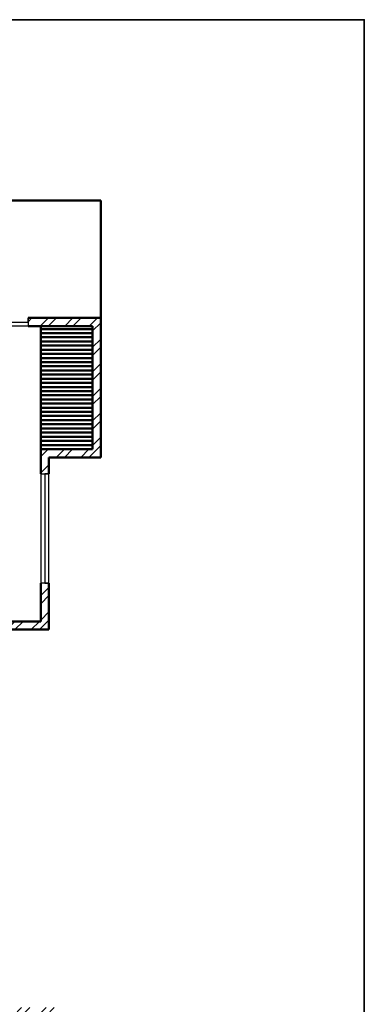
# Model space of a CAD drawing. Units: inches. Extents: x 963 to 2075, y 289 to 2657.
# Tile 98 of 98: x 1885 to 2075, y 2117 to 2657. Entities that reach past the tile are written whole.
import ezdxf

# ---------------------------------------------------------------- set-up
doc = ezdxf.new("R2010")
doc.units = ezdxf.units.IN
for name, color, linetype, lineweight in [('A-ANNO-TTLB', 7, 'Continuous', 35), ('A-GLAZ', 3, 'Continuous', 25), ('A-WALL', 7, 'Continuous', 50), ('A-WALL-PATT', 8, 'Continuous', 13)]:
    doc.layers.add(name, color=color, linetype=linetype, lineweight=lineweight)

msp = doc.modelspace()

# ---------------------------------------------------------------- hatches: boundary and pattern name
at = {"layer": 'A-WALL-PATT'}
h = msp.add_hatch(dxfattribs=at)
h.set_pattern_fill('ANSI32', color=256)
h.paths.add_polyline_path([(1296.92, 2558.32), (1203.92, 2558.32), (1203.92, 2493.82), (1191.53, 2493.82), (1191.53, 2489.32), (1211.06, 2489.32), (1211.06, 2492.02), (1211.06, 2493.82), (1208.42, 2493.82), (1208.42, 2553.82), (1292.42, 2553.82), (1292.42, 2538.86), (1296.92, 2538.86)])
h.paths.add_polyline_path([(1442.42, 2558.32), (1349.42, 2558.32), (1349.42, 2538.94), (1353.92, 2538.94), (1353.92, 2553.82), (1437.92, 2553.82), (1437.92, 2493.82), (1434.54, 2493.82), (1434.54, 2489.32), (1448.31, 2489.32), (1448.31, 2491.57), (1448.31, 2493.82), (1442.42, 2493.82)])
h.paths.add_polyline_path([(1415.55, 2491.57), (1415.55, 2493.82), (1340.94, 2493.82), (1340.94, 2489.32), (1371.92, 2489.32), (1371.92, 2378.32), (1367.6, 2378.32), (1367.6, 2373.82), (1371.92, 2373.82), (1371.92, 2355.19), (1376.42, 2355.19), (1376.42, 2489.32), (1415.55, 2489.32)])
h.paths.add_polyline_path([(1304.94, 2491.57), (1304.94, 2493.82), (1296.92, 2493.82), (1296.92, 2514.86), (1292.42, 2514.86), (1292.42, 2493.82), (1232.81, 2493.82), (1232.81, 2489.32), (1256.42, 2489.32), (1256.42, 2327.32), (1253.71, 2327.32), (1253.71, 2322.82), (1328.42, 2322.82), (1328.42, 2331.15), (1323.92, 2331.15), (1323.92, 2327.32), (1260.92, 2327.32), (1260.92, 2373.82), (1323.92, 2373.82), (1323.92, 2357.81), (1328.42, 2357.81), (1328.42, 2373.82), (1346.01, 2373.82), (1346.01, 2376.07), (1346.01, 2378.32), (1260.92, 2378.32), (1260.92, 2489.32), (1304.94, 2489.32)])
h.paths.add_polyline_path([(1226.65, 2327.32), (1124.42, 2327.32), (1124.42, 2347.45), (1119.92, 2347.45), (1119.92, 2322.82), (1163.42, 2322.82), (1163.42, 2305.43), (1165.67, 2305.43), (1167.92, 2305.43), (1167.92, 2322.82), (1226.65, 2322.82), (1226.65, 2325.07)])
h.paths.add_polyline_path([(1095.92, 2489.32), (1124.42, 2489.32), (1131.53, 2489.32), (1131.53, 2491.57), (1131.53, 2493.82), (1119.92, 2493.82), (1091.42, 2493.82), (1091.42, 2417.32), (1095.92, 2417.32), (1119.92, 2417.32), (1119.92, 2407.45), (1124.42, 2407.45), (1124.42, 2421.82), (1095.92, 2421.82)])
h.paths.add_polyline_path([(1512.92, 2558.32), (1508.42, 2558.32), (1508.42, 2493.82), (1503.4, 2493.82), (1503.4, 2489.32), (1508.42, 2489.32), (1508.42, 2327.32), (1376.42, 2327.32), (1376.42, 2330.27), (1371.92, 2330.27), (1371.92, 2298.74), (1376.42, 2298.74), (1376.42, 2322.82), (1508.42, 2322.82), (1508.42, 2165.32), (1504.26, 2165.32), (1504.26, 2160.82), (1508.42, 2160.82), (1508.42, 2108.32), (1512.92, 2108.32), (1512.92, 2160.82), (1516.18, 2160.82), (1516.18, 2163.07), (1516.18, 2165.32), (1512.92, 2165.32), (1512.92, 2322.82), (1644.92, 2322.82), (1644.92, 2298.74), (1649.42, 2298.74), (1649.42, 2322.82), (1649.42, 2330.94), (1647.17, 2330.94), (1644.92, 2330.94), (1644.92, 2327.32), (1512.92, 2327.32), (1512.92, 2489.32), (1516.76, 2489.32), (1516.76, 2491.57), (1516.76, 2493.82), (1512.92, 2493.82)])
h.paths.add_polyline_path([(1671.92, 2558.32), (1578.92, 2558.32), (1578.92, 2493.82), (1573.53, 2493.82), (1573.53, 2489.32), (1586.54, 2489.32), (1586.54, 2491.57), (1586.54, 2493.82), (1583.42, 2493.82), (1583.42, 2553.82), (1667.42, 2553.82), (1667.42, 2541.11), (1671.92, 2541.11)])
h.paths.add_polyline_path([(1681.26, 2493.82), (1671.92, 2493.82), (1671.92, 2517.11), (1667.42, 2517.11), (1667.42, 2493.82), (1610.22, 2493.82), (1610.22, 2489.32), (1644.92, 2489.32), (1644.92, 2357.87), (1649.42, 2357.87), (1649.42, 2373.82), (1652.2, 2373.82), (1652.2, 2375.83), (1652.2, 2378.32), (1649.42, 2378.32), (1649.42, 2489.32), (1681.26, 2489.32), (1681.26, 2491.57)])
h.paths.add_polyline_path([(1821.92, 2558.32), (1728.92, 2558.32), (1728.92, 2541), (1733.42, 2541), (1733.42, 2553.82), (1817.42, 2553.82), (1817.42, 2493.82), (1813.51, 2493.82), (1813.51, 2489.32), (1830.08, 2489.32), (1830.08, 2491.57), (1830.08, 2493.82), (1821.92, 2493.82)])
h.paths.add_polyline_path([(1794.24, 2493.82), (1717.26, 2493.82), (1717.26, 2489.32), (1760.42, 2489.32), (1760.42, 2378.32), (1674.4, 2378.32), (1674.4, 2373.82), (1692.92, 2373.82), (1692.92, 2356.95), (1697.42, 2356.95), (1697.42, 2373.82), (1760.42, 2373.82), (1760.42, 2327.32), (1697.42, 2327.32), (1697.42, 2333.34), (1692.92, 2333.34), (1692.92, 2322.82), (1768.04, 2322.82), (1768.04, 2325.07), (1768.04, 2327.32), (1764.92, 2327.32), (1764.92, 2489.32), (1794.24, 2489.32)])
h.paths.add_polyline_path([(1733.42, 2517), (1728.92, 2517), (1728.92, 2493.82), (1733.42, 2493.82)], flags=17)
h.paths.add_polyline_path([(1929.92, 2493.82), (1890.08, 2493.82), (1890.08, 2489.32), (1896.92, 2489.32), (1925.42, 2489.32), (1925.42, 2421.82), (1896.92, 2421.82), (1896.92, 2408.32), (1901.42, 2408.32), (1901.42, 2417.32), (1925.42, 2417.32), (1929.92, 2417.32)])
h.paths.add_polyline_path([(1901.42, 2348.32), (1896.92, 2348.32), (1896.92, 2327.32), (1800.42, 2327.32), (1800.42, 2322.82), (1853.42, 2322.82), (1853.42, 2309.45), (1857.92, 2309.45), (1857.92, 2322.82), (1901.42, 2322.82)])
h.paths.add_polyline_path([(1857.92, 2249.45), (1853.42, 2249.45), (1853.42, 2214.82), (1686.31, 2214.82), (1686.31, 2210.32), (1853.42, 2210.32), (1853.42, 2202.13), (1857.92, 2202.13), (1857.92, 2210.32)])
h.paths.add_polyline_path([(1857.92, 2142.13), (1853.42, 2142.13), (1853.42, 2115.42), (1841.42, 2115.42), (1841.42, 2088.53), (1841.42, 2046.95), (1845.92, 2046.95), (1845.92, 2110.92), (1905.92, 2110.92), (1905.92, 2092.52), (1910.42, 2092.52), (1910.42, 2115.42), (1857.92, 2115.42)])
h.paths.add_polyline_path([(1532.44, 1482.34), (1573.46, 1482.34), (1573.46, 1501), (1532.44, 1501)], flags=9)
h.paths.add_polyline_path([(1438.66, 1486.3), (1479.68, 1486.3), (1479.68, 1504.96), (1438.66, 1504.96)], flags=9)
h.paths.add_polyline_path([(1411.22, 1365.31), (1659.14, 1365.31), (1659.14, 1402.4), (1411.22, 1402.4)], flags=9)
h.paths.add_polyline_path([(1185.67, 2296.3), (1248.16, 2296.3), (1248.16, 2314.95), (1185.67, 2314.95)], flags=9)
h.paths.add_polyline_path([(1177.31, 2187.35), (1216.15, 2187.35), (1216.15, 2206.01), (1177.31, 2206.01)], flags=9)
h.paths.add_polyline_path([(1295.1, 1602.08), (1328.26, 1602.08), (1328.26, 1620.74), (1295.1, 1620.74)], flags=9)
h.paths.add_polyline_path([(1525.13, 2005.99), (1558.39, 2005.99), (1558.39, 2024.65), (1525.13, 2024.65)], flags=9)
h.paths.add_polyline_path([(1459.61, 1977.13), (1472.19, 1977.13), (1472.19, 1987.43), (1459.61, 1987.43)], flags=9)
h.paths.add_polyline_path([(1467.81, 2053.68), (1480.02, 2053.68), (1480.02, 2063.98), (1467.81, 2063.98)], flags=9)
h.paths.add_polyline_path([(1555.18, 2119.02), (1584.56, 2119.02), (1584.56, 2137.68), (1555.18, 2137.68)], flags=25)
h.paths.add_polyline_path([(1405.39, 2115.29), (1444.48, 2115.29), (1444.48, 2133.95), (1405.39, 2133.95)], flags=25)
h.paths.add_polyline_path([(1698.48, 2004.26), (1727.69, 2004.26), (1727.69, 2022.92), (1698.48, 2022.92)], flags=9)
h.paths.add_polyline_path([(1612.16, 1972.86), (1629.02, 1972.86), (1629.02, 1983.16), (1612.16, 1983.16)], flags=9)
h.paths.add_polyline_path([(1608.29, 2060.04), (1625.15, 2060.04), (1625.15, 2070.34), (1608.29, 2070.34)], flags=9)
h.paths.add_polyline_path([(1527.95, 1684.4), (1566.79, 1684.4), (1566.79, 1703.06), (1527.95, 1703.06)], flags=9)
h.paths.add_polyline_path([(1422.79, 1683.59), (1461.63, 1683.59), (1461.63, 1702.25), (1422.79, 1702.25)], flags=9)
h.paths.add_polyline_path([(1531.26, 1732.46), (1574.01, 1732.46), (1574.01, 1751.12), (1531.26, 1751.12)], flags=9)
h.paths.add_polyline_path([(1402.87, 1732.85), (1439.8, 1732.85), (1439.8, 1751.5), (1402.87, 1751.5)], flags=9)
h.paths.add_polyline_path([(1243.12, 1923.13), (1281.96, 1923.13), (1281.96, 1941.79), (1243.12, 1941.79)], flags=9)
h.paths.add_polyline_path([(1181.75, 1792.27), (1244.24, 1792.27), (1244.24, 1810.93), (1181.75, 1810.93)], flags=9)
h.paths.add_polyline_path([(1265.82, 1670.3), (1316.07, 1670.3), (1316.07, 1688.96), (1265.82, 1688.96)], flags=9)
h.paths.add_polyline_path([(1140.26, 1676.05), (1179.1, 1676.05), (1179.1, 1694.71), (1140.26, 1694.71)], flags=9)
h.paths.add_polyline_path([(1107.49, 1490.89), (1143.37, 1490.89), (1143.37, 1509.55), (1107.49, 1509.55)], flags=9)
h.paths.add_polyline_path([(1217.58, 1483.9), (1246.74, 1483.9), (1246.74, 1502.56), (1217.58, 1502.56)], flags=9)
h.paths.add_polyline_path([(1389.21, 1486.92), (1418.37, 1486.92), (1418.37, 1505.58), (1389.21, 1505.58)], flags=9)
h.paths.add_polyline_path([(1672.21, 1602.08), (1705.37, 1602.08), (1705.37, 1620.74), (1672.21, 1620.74)], flags=9)
h.paths.add_polyline_path([(1752.08, 1522.64), (1781.24, 1522.64), (1781.24, 1541.3), (1752.08, 1541.3)], flags=9)
h.paths.add_polyline_path([(1848.27, 1491.26), (1884.16, 1491.26), (1884.16, 1509.92), (1848.27, 1509.92)], flags=9)
h.paths.add_polyline_path([(1822.47, 1685.62), (1861.31, 1685.62), (1861.31, 1704.28), (1822.47, 1704.28)], flags=9)
h.paths.add_polyline_path([(1713.19, 1672.23), (1763.44, 1672.23), (1763.44, 1690.89), (1713.19, 1690.89)], flags=9)
h.paths.add_polyline_path([(1736.62, 1790.58), (1799.11, 1790.58), (1799.11, 1809.24), (1736.62, 1809.24)], flags=9)
h.paths.add_polyline_path([(1691.49, 1916.36), (1730.33, 1916.36), (1730.33, 1935.01), (1691.49, 1935.01)], flags=9)
h.paths.add_polyline_path([(1764.87, 1973.92), (1794.31, 1973.92), (1794.31, 1992.58), (1764.87, 1992.58)], flags=9)
h.paths.add_polyline_path([(1767.85, 2034.02), (1797.29, 2034.02), (1797.29, 2052.67), (1767.85, 2052.67)], flags=9)
h.paths.add_polyline_path([(1851.59, 2060.33), (1880.75, 2060.33), (1880.75, 2078.99), (1851.59, 2078.99)], flags=25)
h.paths.add_polyline_path([(1688.49, 2086.87), (1727.33, 2086.87), (1727.33, 2105.53), (1688.49, 2105.53)], flags=9)
h.paths.add_polyline_path([(1537.74, 2293.58), (1580.49, 2293.58), (1580.49, 2312.24), (1537.74, 2312.24)], flags=25)
h.paths.add_polyline_path([(1425.59, 2296.11), (1468.34, 2296.11), (1468.34, 2314.77), (1425.59, 2314.77)], flags=25)
h.paths.add_polyline_path([(1278.52, 2004.18), (1307.72, 2004.18), (1307.72, 2022.84), (1278.52, 2022.84)], flags=9)
h.paths.add_polyline_path([(1193.28, 1973.63), (1222.72, 1973.63), (1222.72, 1992.29), (1193.28, 1992.29)], flags=9)
h.paths.add_polyline_path([(1192.41, 2040.58), (1221.84, 2040.58), (1221.84, 2059.23), (1192.41, 2059.23)], flags=9)
h.paths.add_polyline_path([(1130.6, 1951.39), (1159.76, 1951.39), (1159.76, 1970.05), (1130.6, 1970.05)], flags=9)
h.paths.add_polyline_path([(1132.83, 2052.49), (1161.98, 2052.49), (1161.98, 2071.15), (1132.83, 2071.15)], flags=9)
h.paths.add_polyline_path([(1265.13, 2334.62), (1315.38, 2334.62), (1315.38, 2353.28), (1265.13, 2353.28)], flags=25)
h.paths.add_polyline_path([(1136.74, 2330.79), (1175.58, 2330.79), (1175.58, 2349.44), (1136.74, 2349.44)], flags=9)
h.paths.add_polyline_path([(1287.42, 2417.2), (1320.58, 2417.2), (1320.58, 2435.86), (1287.42, 2435.86)], flags=25)
h.paths.add_polyline_path([(1430.99, 2329.16), (1469.83, 2329.16), (1469.83, 2347.82), (1430.99, 2347.82)], flags=25)
h.paths.add_polyline_path([(1525.42, 2329.21), (1564.26, 2329.21), (1564.26, 2347.87), (1525.42, 2347.87)], flags=25)
h.paths.add_polyline_path([(1684.52, 2382.8), (1717.68, 2382.8), (1717.68, 2401.46), (1684.52, 2401.46)], flags=25)
h.paths.add_polyline_path([(1704.81, 2340.29), (1755.05, 2340.29), (1755.05, 2358.95), (1704.81, 2358.95)], flags=25)
h.paths.add_polyline_path([(1694.11, 2287.76), (1756.6, 2287.76), (1756.6, 2306.41), (1694.11, 2306.41)], flags=9)
h.paths.add_polyline_path([(1815.78, 2329.86), (1854.62, 2329.86), (1854.62, 2348.52), (1815.78, 2348.52)], flags=9)
h.paths.add_polyline_path([(1842.87, 2514.26), (1878.76, 2514.26), (1878.76, 2532.91), (1842.87, 2532.91)], flags=9)
h.paths.add_polyline_path([(1769.51, 2531.45), (1798.67, 2531.45), (1798.67, 2550.1), (1769.51, 2550.1)], flags=25)
h.paths.add_polyline_path([(1594.77, 2518.47), (1623.93, 2518.47), (1623.93, 2537.13), (1594.77, 2537.13)], flags=25)
h.paths.add_polyline_path([(1520.72, 2516.18), (1556.61, 2516.18), (1556.61, 2534.84), (1520.72, 2534.84)], flags=25)
h.paths.add_polyline_path([(1464.46, 2516.69), (1500.34, 2516.69), (1500.34, 2535.35), (1464.46, 2535.35)], flags=25)
h.paths.add_polyline_path([(1365.7, 2528.97), (1394.85, 2528.97), (1394.85, 2547.63), (1365.7, 2547.63)], flags=25)
h.paths.add_polyline_path([(1222.84, 2516.23), (1252, 2516.23), (1252, 2534.89), (1222.84, 2534.89)], flags=25)
h.paths.add_polyline_path([(1104.55, 2509.6), (1140.43, 2509.6), (1140.43, 2528.26), (1104.55, 2528.26)], flags=9)

# ---------------------------------------------------------------- linework, layer by layer
at = {"layer": 'A-ANNO-TTLB'}
msp.add_lwpolyline([(962.81, 2657.49), (2074.6, 2657.49), (2074.6, 1303.08), (962.81, 1303.08)], close=True, dxfattribs=at)
at = {"layer": 'A-GLAZ'}
for p, q in [((1830.08, 2491.57), (1890.08, 2491.57)), ((1890.08, 2491.57), (1890.08, 2493.82)), ((1890.08, 2493.82), (1890.08, 2489.32)), ((1890.08, 2489.32), (1848.98, 2489.32)), ((1896.92, 2408.32), (1901.42, 2408.32)), ((1896.92, 2408.32), (1896.92, 2348.32)), ((1901.42, 2408.32), (1899.17, 2408.32)), ((1899.17, 2408.32), (1899.17, 2348.32)), ((1901.42, 2348.32), (1901.42, 2408.32)), ((1901.42, 2348.32), (1896.92, 2348.32)), ((1899.17, 2348.32), (1901.42, 2348.32))]:
    msp.add_line(p, q, dxfattribs=at)
at = {"layer": 'A-WALL'}
for p, q in [((1728.92, 2558.32), (1929.92, 2558.32)), ((1929.92, 2558.32), (1925.42, 2558.32)), ((1929.92, 2558.32), (1929.92, 2553.82)), ((1929.92, 2493.82), (1929.92, 2553.82)), ((1890.08, 2493.82), (1929.92, 2493.82)), ((1890.08, 2493.82), (1901.42, 2493.82)), ((1929.92, 2417.32), (1929.92, 2493.82)), ((1890.08, 2489.32), (1896.92, 2489.32)), ((1896.92, 2489.32), (1896.92, 2408.32)), ((1896.92, 2489.32), (1925.42, 2489.32)), ((1925.42, 2487.75), (1896.92, 2487.75)), ((1925.42, 2489.32), (1925.42, 2421.82)), ((1925.42, 2485.48), (1896.92, 2485.48)), ((1925.42, 2483.2), (1896.92, 2483.2)), ((1925.42, 2480.93), (1896.92, 2480.93)), ((1925.42, 2478.66), (1896.92, 2478.66)), ((1925.42, 2476.38), (1896.92, 2476.38)), ((1925.42, 2474.11), (1896.92, 2474.11)), ((1925.42, 2471.83), (1896.92, 2471.83)), ((1925.42, 2469.56), (1896.92, 2469.56)), ((1925.42, 2467.29), (1896.92, 2467.29)), ((1925.42, 2465.01), (1896.92, 2465.01)), ((1925.42, 2462.74), (1896.92, 2462.74)), ((1925.42, 2460.47), (1896.92, 2460.47)), ((1925.42, 2458.19), (1896.92, 2458.19)), ((1925.42, 2455.92), (1896.92, 2455.92)), ((1925.42, 2453.65), (1896.92, 2453.65)), ((1925.42, 2451.37), (1896.92, 2451.37)), ((1925.42, 2449.1), (1896.92, 2449.1)), ((1925.42, 2446.83), (1896.92, 2446.83)), ((1925.42, 2444.55), (1896.92, 2444.55)), ((1925.42, 2442.28), (1896.92, 2442.28)), ((1925.42, 2440.01), (1896.92, 2440.01)), ((1925.42, 2437.73), (1896.92, 2437.73)), ((1925.42, 2435.46), (1896.92, 2435.46)), ((1925.42, 2433.19), (1896.92, 2433.19)), ((1925.42, 2430.91), (1896.92, 2430.91)), ((1925.42, 2428.64), (1896.92, 2428.64)), ((1925.42, 2426.36), (1896.92, 2426.36)), ((1925.42, 2424.09), (1896.92, 2424.09)), ((1925.42, 2421.82), (1896.92, 2421.82)), ((1901.42, 2417.32), (1925.42, 2417.32)), ((1901.42, 2417.32), (1901.42, 2408.32)), ((1925.42, 2417.32), (1929.92, 2417.32)), ((1896.92, 2348.32), (1896.92, 2327.32)), ((1901.42, 2348.32), (1901.42, 2322.82)), ((1798.87, 2327.32), (1896.92, 2327.32)), ((1857.92, 2322.82), (1901.42, 2322.82))]:
    msp.add_line(p, q, dxfattribs=at)

doc.saveas('drawing.dxf')
